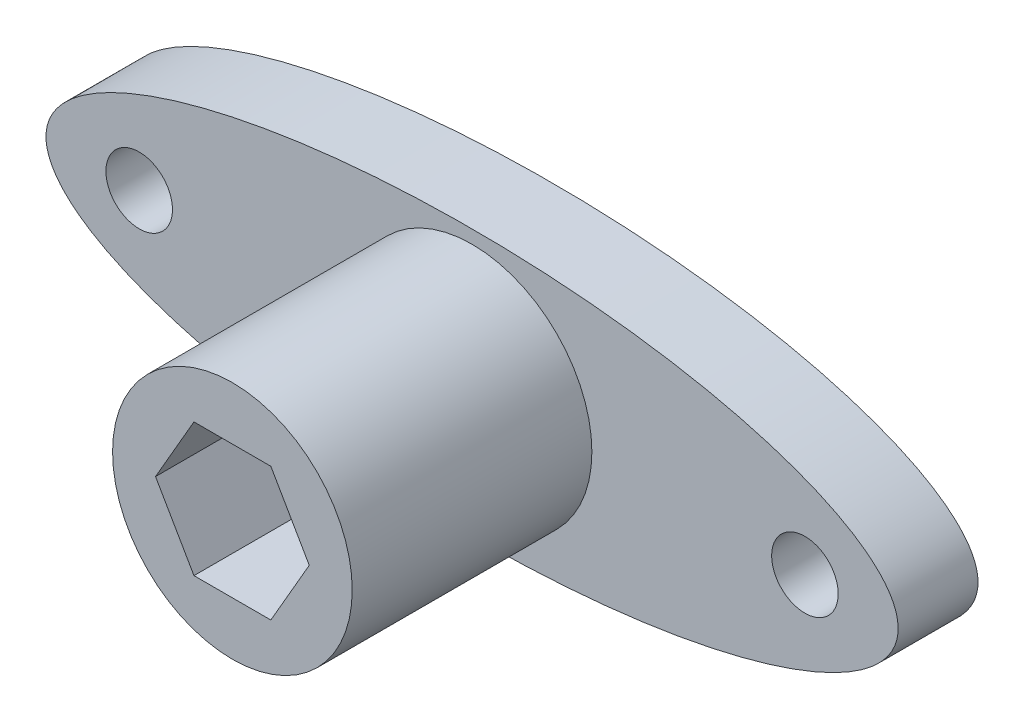
ISO-10303-21;
HEADER;
FILE_DESCRIPTION(('STEP AP214'),'2;1');
FILE_NAME('part.step','',(''),(''),'','','');
FILE_SCHEMA(('AUTOMOTIVE_DESIGN { 1 0 10303 214 1 1 1 1 }'));
ENDSEC;
DATA;
#1=APPLICATION_CONTEXT('core data for automotive mechanical design processes');
#2=APPLICATION_PROTOCOL_DEFINITION('international standard','automotive_design',2000,#1);
#3=PRODUCT_CONTEXT('',#1,'mechanical');
#4=PRODUCT('Part','Part','',(#3));
#5=PRODUCT_RELATED_PRODUCT_CATEGORY('part','',(#4));
#6=PRODUCT_DEFINITION_FORMATION('','',#4);
#7=PRODUCT_DEFINITION_CONTEXT('part definition',#1,'design');
#8=PRODUCT_DEFINITION('design','',#6,#7);
#9=PRODUCT_DEFINITION_SHAPE('','',#8);
#10=(LENGTH_UNIT() NAMED_UNIT(*) SI_UNIT(.MILLI.,.METRE.));
#11=(NAMED_UNIT(*) PLANE_ANGLE_UNIT() SI_UNIT($,.RADIAN.));
#12=(NAMED_UNIT(*) SI_UNIT($,.STERADIAN.) SOLID_ANGLE_UNIT());
#13=UNCERTAINTY_MEASURE_WITH_UNIT(LENGTH_MEASURE(1.E-05),#10,'distance_accuracy_value','');
#14=(GEOMETRIC_REPRESENTATION_CONTEXT(3) GLOBAL_UNCERTAINTY_ASSIGNED_CONTEXT((#13)) GLOBAL_UNIT_ASSIGNED_CONTEXT((#10,
#11,#12)) REPRESENTATION_CONTEXT('',''));
#15=CARTESIAN_POINT('',(0.,0.,0.));
#16=DIRECTION('',(0.,0.,1.));
#17=DIRECTION('',(1.,0.,0.));
#18=AXIS2_PLACEMENT_3D('',#15,#16,#17);
#19=CARTESIAN_POINT('',(0.,0.,0.15));
#20=DIRECTION('',(0.,0.,1.));
#21=DIRECTION('',(1.,0.,0.));
#22=AXIS2_PLACEMENT_3D('',#19,#20,#21);
#23=ELLIPSE('',#22,0.8,0.25);
#24=DIRECTION('',(0.,0.,-1.));
#25=VECTOR('',#24,1.);
#26=SURFACE_OF_LINEAR_EXTRUSION('',#23,#25);
#27=CARTESIAN_POINT('',(0.8,0.,0.15));
#28=VERTEX_POINT('',#27);
#29=EDGE_CURVE('E11',#28,#28,#23,.T.);
#30=ORIENTED_EDGE('',*,*,#29,.F.);
#31=EDGE_LOOP('',(#30));
#32=FACE_BOUND('',#31,.T.);
#33=CARTESIAN_POINT('',(0.,0.,0.));
#34=DIRECTION('',(0.,0.,1.));
#35=DIRECTION('',(1.,0.,0.));
#36=AXIS2_PLACEMENT_3D('',#33,#34,#35);
#37=ELLIPSE('',#36,0.8,0.25);
#38=CARTESIAN_POINT('',(0.8,0.,0.));
#39=VERTEX_POINT('',#38);
#40=EDGE_CURVE('E43',#39,#39,#37,.T.);
#41=ORIENTED_EDGE('',*,*,#40,.T.);
#42=EDGE_LOOP('',(#41));
#43=FACE_BOUND('',#42,.T.);
#44=ADVANCED_FACE('F39',(#32,#43),#26,.F.);
#45=CARTESIAN_POINT('',(0.,0.,0.15));
#46=DIRECTION('',(0.,0.,1.));
#47=DIRECTION('',(1.,0.,0.));
#48=AXIS2_PLACEMENT_3D('',#45,#46,#47);
#49=PLANE('',#48);
#50=CARTESIAN_POINT('',(0.624999999999987,0.,0.15));
#51=DIRECTION('',(0.,0.,-1.));
#52=DIRECTION('',(-1.,0.,0.));
#53=AXIS2_PLACEMENT_3D('',#50,#51,#52);
#54=CIRCLE('',#53,0.0625000000000001);
#55=CARTESIAN_POINT('',(0.562499999999987,0.,0.15));
#56=VERTEX_POINT('',#55);
#57=EDGE_CURVE('E126',#56,#56,#54,.T.);
#58=ORIENTED_EDGE('',*,*,#57,.T.);
#59=EDGE_LOOP('',(#58));
#60=FACE_BOUND('',#59,.T.);
#61=CARTESIAN_POINT('',(-0.625,0.,0.15));
#62=DIRECTION('',(0.,0.,-1.));
#63=DIRECTION('',(-1.,0.,0.));
#64=AXIS2_PLACEMENT_3D('',#61,#62,#63);
#65=CIRCLE('',#64,0.0625000000000001);
#66=CARTESIAN_POINT('',(-0.6875,0.,0.15));
#67=VERTEX_POINT('',#66);
#68=EDGE_CURVE('E222',#67,#67,#65,.T.);
#69=ORIENTED_EDGE('',*,*,#68,.T.);
#70=EDGE_LOOP('',(#69));
#71=FACE_BOUND('',#70,.T.);
#72=CARTESIAN_POINT('',(0.,0.,0.15));
#73=DIRECTION('',(0.,0.,1.));
#74=DIRECTION('',(1.,0.,0.));
#75=AXIS2_PLACEMENT_3D('',#72,#73,#74);
#76=CIRCLE('',#75,0.225);
#77=CARTESIAN_POINT('',(0.225,0.,0.15));
#78=VERTEX_POINT('',#77);
#79=EDGE_CURVE('E143',#78,#78,#76,.T.);
#80=ORIENTED_EDGE('',*,*,#79,.F.);
#81=EDGE_LOOP('',(#80));
#82=FACE_BOUND('',#81,.T.);
#83=ORIENTED_EDGE('',*,*,#29,.T.);
#84=EDGE_LOOP('',(#83));
#85=FACE_BOUND('',#84,.T.);
#86=ADVANCED_FACE('F156',(#60,#71,#82,#85),#49,.T.);
#87=CARTESIAN_POINT('',(0.,0.,0.));
#88=DIRECTION('',(0.,0.,1.));
#89=DIRECTION('',(1.,0.,0.));
#90=AXIS2_PLACEMENT_3D('',#87,#88,#89);
#91=PLANE('',#90);
#92=CARTESIAN_POINT('',(0.624999999999987,0.,0.));
#93=DIRECTION('',(0.,0.,-1.));
#94=DIRECTION('',(-1.,0.,0.));
#95=AXIS2_PLACEMENT_3D('',#92,#93,#94);
#96=CIRCLE('',#95,0.0625000000000001);
#97=CARTESIAN_POINT('',(0.562499999999987,0.,0.));
#98=VERTEX_POINT('',#97);
#99=EDGE_CURVE('E216',#98,#98,#96,.T.);
#100=ORIENTED_EDGE('',*,*,#99,.F.);
#101=EDGE_LOOP('',(#100));
#102=FACE_BOUND('',#101,.T.);
#103=CARTESIAN_POINT('',(-0.625,0.,0.));
#104=DIRECTION('',(0.,0.,-1.));
#105=DIRECTION('',(-1.,0.,0.));
#106=AXIS2_PLACEMENT_3D('',#103,#104,#105);
#107=CIRCLE('',#106,0.0625000000000001);
#108=CARTESIAN_POINT('',(-0.6875,0.,0.));
#109=VERTEX_POINT('',#108);
#110=EDGE_CURVE('E220',#109,#109,#107,.T.);
#111=ORIENTED_EDGE('',*,*,#110,.F.);
#112=EDGE_LOOP('',(#111));
#113=FACE_BOUND('',#112,.T.);
#114=ORIENTED_EDGE('',*,*,#40,.F.);
#115=EDGE_LOOP('',(#114));
#116=FACE_BOUND('',#115,.T.);
#117=ADVANCED_FACE('F157',(#102,#113,#116),#91,.F.);
#118=CARTESIAN_POINT('',(0.,0.,0.6));
#119=DIRECTION('',(0.,0.,-1.));
#120=DIRECTION('',(-1.,0.,0.));
#121=AXIS2_PLACEMENT_3D('',#118,#119,#120);
#122=CYLINDRICAL_SURFACE('',#121,0.225);
#123=CARTESIAN_POINT('',(0.,0.,0.6));
#124=DIRECTION('',(0.,0.,1.));
#125=DIRECTION('',(1.,0.,0.));
#126=AXIS2_PLACEMENT_3D('',#123,#124,#125);
#127=CIRCLE('',#126,0.225);
#128=CARTESIAN_POINT('',(0.225,0.,0.6));
#129=VERTEX_POINT('',#128);
#130=EDGE_CURVE('E150',#129,#129,#127,.T.);
#131=ORIENTED_EDGE('',*,*,#130,.F.);
#132=EDGE_LOOP('',(#131));
#133=FACE_BOUND('',#132,.T.);
#134=ORIENTED_EDGE('',*,*,#79,.T.);
#135=EDGE_LOOP('',(#134));
#136=FACE_BOUND('',#135,.T.);
#137=ADVANCED_FACE('F152',(#133,#136),#122,.T.);
#138=CARTESIAN_POINT('',(0.,0.,0.6));
#139=DIRECTION('',(0.,0.,1.));
#140=DIRECTION('',(1.,0.,0.));
#141=AXIS2_PLACEMENT_3D('',#138,#139,#140);
#142=PLANE('',#141);
#143=DIRECTION('',(-0.5,-0.866025403784438,0.));
#144=VECTOR('',#143,1.);
#145=CARTESIAN_POINT('',(-0.0721687836487032,0.125,0.6));
#146=LINE('',#145,#144);
#147=CARTESIAN_POINT('',(-0.0721687836487032,0.125,0.6));
#148=VERTEX_POINT('',#147);
#149=CARTESIAN_POINT('',(-0.144337567297406,0.,0.6));
#150=VERTEX_POINT('',#149);
#151=EDGE_CURVE('E52',#148,#150,#146,.T.);
#152=ORIENTED_EDGE('',*,*,#151,.F.);
#153=DIRECTION('',(-1.,0.,0.));
#154=VECTOR('',#153,1.);
#155=CARTESIAN_POINT('',(0.0721687836487032,0.125,0.6));
#156=LINE('',#155,#154);
#157=CARTESIAN_POINT('',(0.0721687836487032,0.125,0.6));
#158=VERTEX_POINT('',#157);
#159=EDGE_CURVE('E139',#158,#148,#156,.T.);
#160=ORIENTED_EDGE('',*,*,#159,.F.);
#161=DIRECTION('',(-0.5,0.866025403784438,0.));
#162=VECTOR('',#161,1.);
#163=CARTESIAN_POINT('',(0.144337567297407,0.,0.6));
#164=LINE('',#163,#162);
#165=CARTESIAN_POINT('',(0.144337567297407,0.,0.6));
#166=VERTEX_POINT('',#165);
#167=EDGE_CURVE('E134',#166,#158,#164,.T.);
#168=ORIENTED_EDGE('',*,*,#167,.F.);
#169=DIRECTION('',(0.5,0.866025403784438,0.));
#170=VECTOR('',#169,1.);
#171=CARTESIAN_POINT('',(0.0721687836487033,-0.125,0.6));
#172=LINE('',#171,#170);
#173=CARTESIAN_POINT('',(0.0721687836487033,-0.125,0.6));
#174=VERTEX_POINT('',#173);
#175=EDGE_CURVE('E101',#174,#166,#172,.T.);
#176=ORIENTED_EDGE('',*,*,#175,.F.);
#177=DIRECTION('',(1.,0.,0.));
#178=VECTOR('',#177,1.);
#179=CARTESIAN_POINT('',(-0.0721687836487032,-0.125,0.6));
#180=LINE('',#179,#178);
#181=CARTESIAN_POINT('',(-0.0721687836487032,-0.125,0.6));
#182=VERTEX_POINT('',#181);
#183=EDGE_CURVE('E131',#182,#174,#180,.T.);
#184=ORIENTED_EDGE('',*,*,#183,.F.);
#185=DIRECTION('',(0.5,-0.866025403784439,0.));
#186=VECTOR('',#185,1.);
#187=CARTESIAN_POINT('',(-0.144337567297406,0.,0.6));
#188=LINE('',#187,#186);
#189=EDGE_CURVE('E130',#150,#182,#188,.T.);
#190=ORIENTED_EDGE('',*,*,#189,.F.);
#191=EDGE_LOOP('',(#152,#160,#168,#176,#184,#190));
#192=FACE_BOUND('',#191,.T.);
#193=ORIENTED_EDGE('',*,*,#130,.T.);
#194=EDGE_LOOP('',(#193));
#195=FACE_BOUND('',#194,.T.);
#196=ADVANCED_FACE('F174',(#192,#195),#142,.T.);
#197=CARTESIAN_POINT('',(-0.0721687836487032,0.125,0.3));
#198=DIRECTION('',(-0.866025403784439,0.5,0.));
#199=DIRECTION('',(-0.5,-0.866025403784439,0.));
#200=AXIS2_PLACEMENT_3D('',#197,#198,#199);
#201=PLANE('',#200);
#202=ORIENTED_EDGE('',*,*,#151,.T.);
#203=DIRECTION('',(0.,0.,1.));
#204=VECTOR('',#203,1.);
#205=CARTESIAN_POINT('',(-0.144337567297406,0.,0.3));
#206=LINE('',#205,#204);
#207=CARTESIAN_POINT('',(-0.144337567297406,0.,0.3));
#208=VERTEX_POINT('',#207);
#209=EDGE_CURVE('E82',#208,#150,#206,.T.);
#210=ORIENTED_EDGE('',*,*,#209,.F.);
#211=DIRECTION('',(-0.5,-0.866025403784438,0.));
#212=VECTOR('',#211,1.);
#213=CARTESIAN_POINT('',(-0.0721687836487032,0.125,0.3));
#214=LINE('',#213,#212);
#215=CARTESIAN_POINT('',(-0.0721687836487032,0.125,0.3));
#216=VERTEX_POINT('',#215);
#217=EDGE_CURVE('E140',#216,#208,#214,.T.);
#218=ORIENTED_EDGE('',*,*,#217,.F.);
#219=DIRECTION('',(0.,0.,1.));
#220=VECTOR('',#219,1.);
#221=CARTESIAN_POINT('',(-0.0721687836487032,0.125,0.3));
#222=LINE('',#221,#220);
#223=EDGE_CURVE('E61',#216,#148,#222,.T.);
#224=ORIENTED_EDGE('',*,*,#223,.T.);
#225=EDGE_LOOP('',(#202,#210,#218,#224));
#226=FACE_BOUND('',#225,.T.);
#227=ADVANCED_FACE('F181',(#226),#201,.F.);
#228=CARTESIAN_POINT('',(0.0721687836487032,0.125,0.3));
#229=DIRECTION('',(0.,1.,0.));
#230=DIRECTION('',(0.,0.,1.));
#231=AXIS2_PLACEMENT_3D('',#228,#229,#230);
#232=PLANE('',#231);
#233=ORIENTED_EDGE('',*,*,#159,.T.);
#234=ORIENTED_EDGE('',*,*,#223,.F.);
#235=DIRECTION('',(-1.,0.,0.));
#236=VECTOR('',#235,1.);
#237=CARTESIAN_POINT('',(0.0721687836487032,0.125,0.3));
#238=LINE('',#237,#236);
#239=CARTESIAN_POINT('',(0.0721687836487032,0.125,0.3));
#240=VERTEX_POINT('',#239);
#241=EDGE_CURVE('E114',#240,#216,#238,.T.);
#242=ORIENTED_EDGE('',*,*,#241,.F.);
#243=DIRECTION('',(0.,0.,1.));
#244=VECTOR('',#243,1.);
#245=CARTESIAN_POINT('',(0.0721687836487032,0.125,0.3));
#246=LINE('',#245,#244);
#247=EDGE_CURVE('E104',#240,#158,#246,.T.);
#248=ORIENTED_EDGE('',*,*,#247,.T.);
#249=EDGE_LOOP('',(#233,#234,#242,#248));
#250=FACE_BOUND('',#249,.T.);
#251=ADVANCED_FACE('F190',(#250),#232,.F.);
#252=CARTESIAN_POINT('',(0.144337567297407,0.,0.3));
#253=DIRECTION('',(0.866025403784438,0.5,0.));
#254=DIRECTION('',(-0.5,0.866025403784439,0.));
#255=AXIS2_PLACEMENT_3D('',#252,#253,#254);
#256=PLANE('',#255);
#257=ORIENTED_EDGE('',*,*,#167,.T.);
#258=ORIENTED_EDGE('',*,*,#247,.F.);
#259=DIRECTION('',(-0.5,0.866025403784438,0.));
#260=VECTOR('',#259,1.);
#261=CARTESIAN_POINT('',(0.144337567297407,0.,0.3));
#262=LINE('',#261,#260);
#263=CARTESIAN_POINT('',(0.144337567297407,0.,0.3));
#264=VERTEX_POINT('',#263);
#265=EDGE_CURVE('E108',#264,#240,#262,.T.);
#266=ORIENTED_EDGE('',*,*,#265,.F.);
#267=DIRECTION('',(0.,0.,1.));
#268=VECTOR('',#267,1.);
#269=CARTESIAN_POINT('',(0.144337567297407,0.,0.3));
#270=LINE('',#269,#268);
#271=EDGE_CURVE('E94',#264,#166,#270,.T.);
#272=ORIENTED_EDGE('',*,*,#271,.T.);
#273=EDGE_LOOP('',(#257,#258,#266,#272));
#274=FACE_BOUND('',#273,.T.);
#275=ADVANCED_FACE('F109',(#274),#256,.F.);
#276=CARTESIAN_POINT('',(0.0721687836487033,-0.125,0.3));
#277=DIRECTION('',(0.866025403784438,-0.5,0.));
#278=DIRECTION('',(0.5,0.866025403784439,0.));
#279=AXIS2_PLACEMENT_3D('',#276,#277,#278);
#280=PLANE('',#279);
#281=ORIENTED_EDGE('',*,*,#175,.T.);
#282=ORIENTED_EDGE('',*,*,#271,.F.);
#283=DIRECTION('',(0.5,0.866025403784438,0.));
#284=VECTOR('',#283,1.);
#285=CARTESIAN_POINT('',(0.0721687836487033,-0.125,0.3));
#286=LINE('',#285,#284);
#287=CARTESIAN_POINT('',(0.0721687836487033,-0.125,0.3));
#288=VERTEX_POINT('',#287);
#289=EDGE_CURVE('E98',#288,#264,#286,.T.);
#290=ORIENTED_EDGE('',*,*,#289,.F.);
#291=DIRECTION('',(0.,0.,1.));
#292=VECTOR('',#291,1.);
#293=CARTESIAN_POINT('',(0.0721687836487033,-0.125,0.3));
#294=LINE('',#293,#292);
#295=EDGE_CURVE('E106',#288,#174,#294,.T.);
#296=ORIENTED_EDGE('',*,*,#295,.T.);
#297=EDGE_LOOP('',(#281,#282,#290,#296));
#298=FACE_BOUND('',#297,.T.);
#299=ADVANCED_FACE('F96',(#298),#280,.F.);
#300=CARTESIAN_POINT('',(-0.0721687836487032,-0.125,0.3));
#301=DIRECTION('',(0.,-1.,0.));
#302=DIRECTION('',(1.,0.,0.));
#303=AXIS2_PLACEMENT_3D('',#300,#301,#302);
#304=PLANE('',#303);
#305=ORIENTED_EDGE('',*,*,#183,.T.);
#306=ORIENTED_EDGE('',*,*,#295,.F.);
#307=DIRECTION('',(1.,0.,0.));
#308=VECTOR('',#307,1.);
#309=CARTESIAN_POINT('',(-0.0721687836487032,-0.125,0.3));
#310=LINE('',#309,#308);
#311=CARTESIAN_POINT('',(-0.0721687836487032,-0.125,0.3));
#312=VERTEX_POINT('',#311);
#313=EDGE_CURVE('E118',#312,#288,#310,.T.);
#314=ORIENTED_EDGE('',*,*,#313,.F.);
#315=DIRECTION('',(0.,0.,1.));
#316=VECTOR('',#315,1.);
#317=CARTESIAN_POINT('',(-0.0721687836487032,-0.125,0.3));
#318=LINE('',#317,#316);
#319=EDGE_CURVE('E145',#312,#182,#318,.T.);
#320=ORIENTED_EDGE('',*,*,#319,.T.);
#321=EDGE_LOOP('',(#305,#306,#314,#320));
#322=FACE_BOUND('',#321,.T.);
#323=ADVANCED_FACE('F193',(#322),#304,.F.);
#324=CARTESIAN_POINT('',(-0.144337567297406,0.,0.3));
#325=DIRECTION('',(-0.866025403784439,-0.5,0.));
#326=DIRECTION('',(0.5,-0.866025403784439,0.));
#327=AXIS2_PLACEMENT_3D('',#324,#325,#326);
#328=PLANE('',#327);
#329=ORIENTED_EDGE('',*,*,#189,.T.);
#330=ORIENTED_EDGE('',*,*,#319,.F.);
#331=DIRECTION('',(0.5,-0.866025403784439,0.));
#332=VECTOR('',#331,1.);
#333=CARTESIAN_POINT('',(-0.144337567297406,0.,0.3));
#334=LINE('',#333,#332);
#335=EDGE_CURVE('E123',#208,#312,#334,.T.);
#336=ORIENTED_EDGE('',*,*,#335,.F.);
#337=ORIENTED_EDGE('',*,*,#209,.T.);
#338=EDGE_LOOP('',(#329,#330,#336,#337));
#339=FACE_BOUND('',#338,.T.);
#340=ADVANCED_FACE('F187',(#339),#328,.F.);
#341=CARTESIAN_POINT('',(0.,0.,0.3));
#342=DIRECTION('',(0.,0.,1.));
#343=DIRECTION('',(1.,0.,0.));
#344=AXIS2_PLACEMENT_3D('',#341,#342,#343);
#345=PLANE('',#344);
#346=ORIENTED_EDGE('',*,*,#217,.T.);
#347=ORIENTED_EDGE('',*,*,#335,.T.);
#348=ORIENTED_EDGE('',*,*,#313,.T.);
#349=ORIENTED_EDGE('',*,*,#289,.T.);
#350=ORIENTED_EDGE('',*,*,#265,.T.);
#351=ORIENTED_EDGE('',*,*,#241,.T.);
#352=EDGE_LOOP('',(#346,#347,#348,#349,#350,#351));
#353=FACE_BOUND('',#352,.T.);
#354=ADVANCED_FACE('F116',(#353),#345,.T.);
#355=CARTESIAN_POINT('',(-0.625,0.,0.15));
#356=DIRECTION('',(0.,0.,-1.));
#357=DIRECTION('',(-1.,0.,0.));
#358=AXIS2_PLACEMENT_3D('',#355,#356,#357);
#359=CYLINDRICAL_SURFACE('',#358,0.0625000000000001);
#360=ORIENTED_EDGE('',*,*,#68,.F.);
#361=EDGE_LOOP('',(#360));
#362=FACE_BOUND('',#361,.T.);
#363=ORIENTED_EDGE('',*,*,#110,.T.);
#364=EDGE_LOOP('',(#363));
#365=FACE_BOUND('',#364,.T.);
#366=ADVANCED_FACE('F204',(#362,#365),#359,.F.);
#367=CARTESIAN_POINT('',(0.624999999999987,0.,0.15));
#368=DIRECTION('',(0.,0.,-1.));
#369=DIRECTION('',(-1.,0.,0.));
#370=AXIS2_PLACEMENT_3D('',#367,#368,#369);
#371=CYLINDRICAL_SURFACE('',#370,0.0625000000000001);
#372=ORIENTED_EDGE('',*,*,#57,.F.);
#373=EDGE_LOOP('',(#372));
#374=FACE_BOUND('',#373,.T.);
#375=ORIENTED_EDGE('',*,*,#99,.T.);
#376=EDGE_LOOP('',(#375));
#377=FACE_BOUND('',#376,.T.);
#378=ADVANCED_FACE('F206',(#374,#377),#371,.F.);
#379=CLOSED_SHELL('',(#44,#86,#117,#137,#196,#227,#251,#275,#299,#323,#340,#354,#366,#378));
#380=MANIFOLD_SOLID_BREP('B2',#379);
#381=ADVANCED_BREP_SHAPE_REPRESENTATION('',(#18,#380),#14);
#382=SHAPE_DEFINITION_REPRESENTATION(#9,#381);
ENDSEC;
END-ISO-10303-21;
